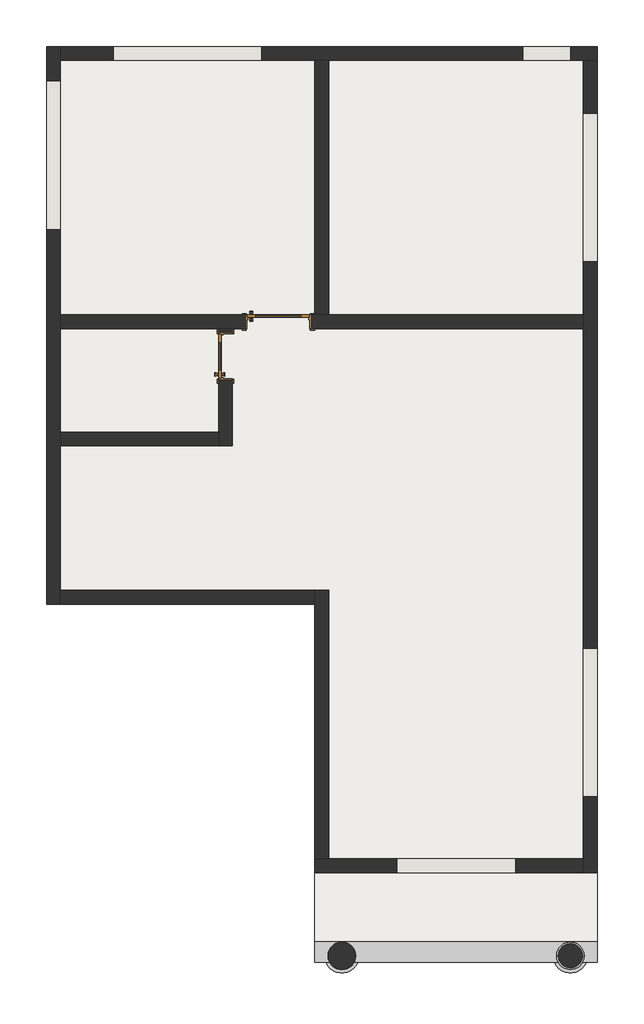
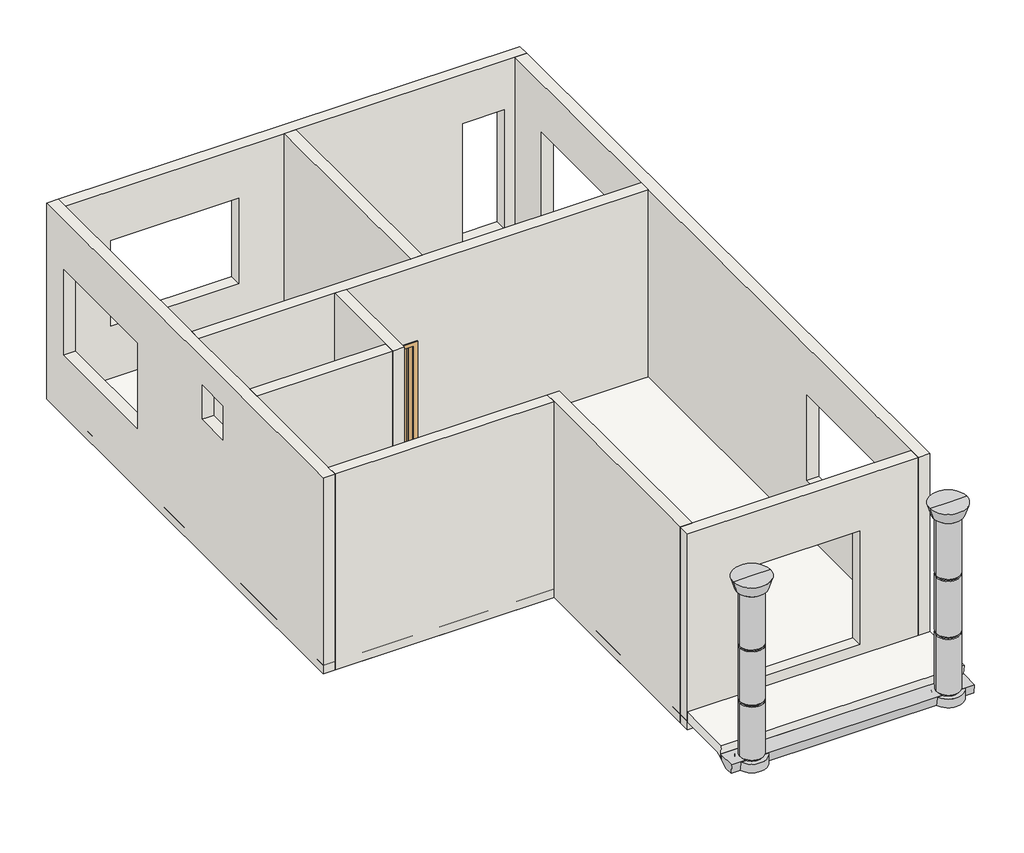
# One storey: 10 walls, 2 columns, 2 doors, 2 slabs, 1 stair flight.
"""IFC4 building model written with IfcOpenShell, lengths in millimetres."""

from ifc_helpers import new_model, si_unit, frame, origin, place, context, project, spatial, polyline, outline, extrude, faceted_brep, transform, mapped, element, save
from components import metal_clad_column_400mm_column_f648cdbd, metal_clad_column_400mm_column_d615f8bc, door_3f7a11fd, door_interior_single_5_panel_vert_wood_650_x_2100_a7f2c8da

model = new_model("IFC4")

# Units and contexts
model_context = context("Model", 3, world=origin())
ifc_project = project(units=[si_unit("LENGTHUNIT", "METRE", prefix="MILLI")], contexts=[model_context])

# Site, building, storey
site = spatial("IfcSite", under=ifc_project)
building = spatial("IfcBuilding", under=site)
storey = spatial("IfcBuildingStorey", under=building, Elevation=-100.0)

# Columns
placement = place(None, origin())
metal_clad_column_400mm_column_shape = metal_clad_column_400mm_column_f648cdbd(model_context)
element("IfcColumn", 1, ObjectType="Metal Clad Column : 400MM COLUMN", at=placement, inside=storey, context=model_context, shape_type="MappedRepresentation", body=[
    mapped(metal_clad_column_400mm_column_shape, transform((-1050.7658003, -5475.1432863, 0.0), x_axis=(1.0, 0.0, 0.0), y_axis=(0.0, 1.0, 0.0), z_axis=(0.0, 0.0, 1.0))),
])
metal_clad_column_400mm_column_2_shape = metal_clad_column_400mm_column_d615f8bc(model_context)
element("IfcColumn", 2, ObjectType="Metal Clad Column : 400MM COLUMN", at=placement, inside=storey, context=model_context, shape_type="MappedRepresentation", body=[
    mapped(metal_clad_column_400mm_column_2_shape, transform((2269.2341997, -5475.1432863, 0.0), x_axis=(-1.0, 0.0, 0.0), y_axis=(0.0, -1.0, 0.0), z_axis=(0.0, 0.0, 1.0))),
])

# Doors
door_shape = door_3f7a11fd(model_context)
element("IfcDoor", 3, ObjectType="Door-Interior-Single-5_Panel_Vert-Wood : 36\" x 82.5\"", at=placement, inside=storey, context=model_context, shape_type="MappedRepresentation", body=[
    mapped(door_shape, transform((-1973.3658003, 3738.0317137, -100.0), x_axis=(1.0, 0.0, 0.0), y_axis=(0.0, 1.0, 0.0), z_axis=(0.0, 0.0, 1.0))),
])
door_interior_single_5_panel_vert_wood_650_x_2100_shape = door_interior_single_5_panel_vert_wood_650_x_2100_a7f2c8da(model_context)
element("IfcDoor", 4, ObjectType="Door-Interior-Single-5_Panel_Vert-Wood : 650 x 2100", at=placement, inside=storey, context=model_context, shape_type="MappedRepresentation", body=[
    mapped(door_interior_single_5_panel_vert_wood_650_x_2100_shape, transform((-2743.9408003, 3234.4567137, -100.0), x_axis=(0.0, 1.0, 0.0), y_axis=(-1.0, 0.0, 0.0), z_axis=(0.0, 0.0, 1.0))),
])

# Slabs
element("IfcSlab", 5, ObjectType="6\" floor", at=placement, inside=storey, context=model_context, shape_type="SweptSolid", body=[
    extrude(outline(polyline([(-5340.7658003, 7734.8567137), (2659.2341997, 7734.8567137), (2659.2341997, -4265.1432863), (-1440.7658003, -4265.1432863), (-1440.7658003, -365.1432863), (-5340.7658003, -365.1432863), (-5340.7658003, 7734.8567137)])), frame((0.0, 0.0, -100.0), z_axis=(0.0, 0.0, 1.0), x_axis=(1.0, 0.0, 0.0)), (0.0, 0.0, 1.0), 150.0),
])
element("IfcSlab", 6, ObjectType="7\" Thickness", at=placement, inside=storey, context=model_context, shape_type="Brep", body=[
    faceted_brep([(2659.2341997, -4265.1432863, 216.6666667), (-1440.7658003, -4265.1432863, 216.6666667), (-1440.7658003, -5145.8176043, 216.6666667), (-1440.7658003, -5265.1432863, 216.6666667), (2659.2341997, -5265.1432863, 216.6666667), (2659.2341997, -5145.8176043, 216.6666667), (2659.2341997, -5246.0932863, 58.3333333), (2659.2341997, -5246.0932863, -13.2231725), (2659.2341997, -5145.8176043, 38.8666667), (2659.2341997, -4265.1432863, 38.8666667), (-1440.7658003, -4265.1432863, 38.8666667), (-1440.7658003, -5246.0932863, 58.3333333), (-1440.7658003, -5145.8176043, 38.8666667), (-1440.7658003, -5246.0932863, -13.2231725)], [[[0, 1, 2, 3, 4, 5]], [[4, 6, 7, 8, 9, 0, 5]], [[1, 0, 9, 10]], [[11, 3, 2, 1, 10, 12, 13]], [[8, 12, 10, 9]], [[4, 3, 11, 6]], [[6, 11, 13, 7]], [[12, 8, 7, 13]]]),
])

# Stair flight
element("IfcStairFlight", 7, ObjectType="3/4\" Nosing", at=placement, inside=storey, context=model_context, shape_type="Brep", body=[
    faceted_brep([(2659.2341997, -5569.9432863, 58.3333333), (-1440.7658003, -5569.9432863, 58.3333333), (-1440.7658003, -5550.8932863, -100.0), (2659.2341997, -5550.8932863, -100.0), (-1440.7658003, -5246.0932863, 58.3333333), (-1440.7658003, -5265.1432863, 58.3333333), (2659.2341997, -5265.1432863, 58.3333333), (2659.2341997, -5246.0932863, 58.3333333), (-1440.7658003, -5246.0932863, -13.2231725), (-1440.7658003, -5265.1432863, -23.1190058), (2659.2341997, -5413.1432464, -100.0), (2659.2341997, -5265.1432863, -23.1190058), (2659.2341997, -5246.0932863, -13.2231725), (-1440.7658003, -5413.1432464, -100.0)], [[[0, 1, 2, 3]], [[4, 5, 1, 0, 6, 7]], [[5, 4, 8, 9]], [[6, 0, 3, 10, 11]], [[4, 7, 12, 8]], [[3, 2, 13, 10]], [[10, 13, 9, 8, 12, 11]], [[1, 5, 9, 13, 2]], [[7, 6, 11, 12]]]),
])

# Walls
element("IfcWall", 8, ObjectType="9\" wall", at=placement, inside=storey, context=model_context, shape_type="Brep", body=[
    faceted_brep([(-5140.7658003, -365.1432863, -100.0), (-5140.7658003, -165.1432863, -100.0), (-5140.7658003, 1934.8567137, -100.0), (-5140.7658003, 2134.8567137, -100.0), (-5140.7658003, 3634.8567137, -100.0), (-5140.7658003, 3834.8567137, -100.0), (-5140.7658003, 7534.8567137, -100.0), (-5140.7658003, 7734.8567137, -100.0), (-5140.7658003, 7734.8567137, 3400.0), (-5140.7658003, 7534.8567137, 3400.0), (-5140.7658003, 3834.8567137, 3400.0), (-5140.7658003, 3634.8567137, 3400.0), (-5140.7658003, 2134.8567137, 3400.0), (-5140.7658003, 1934.8567137, 3400.0), (-5140.7658003, -165.1432863, 3400.0), (-5140.7658003, -365.1432863, 3400.0), (-5140.7658003, 7234.8567137, 2512.7), (-5140.7658003, 7234.8567137, 988.7), (-5140.7658003, 5075.8567137, 988.7), (-5140.7658003, 5075.8567137, 2512.7), (-5140.7658003, 3180.1317137, 2909.6), (-5140.7658003, 3180.1317137, 2300.0), (-5140.7658003, 2570.5317137, 2300.0), (-5140.7658003, 2570.5317137, 2909.6), (-5340.7658003, -365.1432863, -100.0), (-5340.7658003, -365.1432863, 3400.0), (-5340.7658003, 7734.8567137, 3400.0), (-5340.7658003, 7734.8567137, -100.0), (-5340.7658003, 7234.8567137, 2512.7), (-5340.7658003, 5075.8567137, 2512.7), (-5340.7658003, 5075.8567137, 988.7), (-5340.7658003, 7234.8567137, 988.7), (-5340.7658003, 3180.1317137, 2909.6), (-5340.7658003, 2570.5317137, 2909.6), (-5340.7658003, 2570.5317137, 2300.0), (-5340.7658003, 3180.1317137, 2300.0)], [[[0, 1, 2, 3, 4, 5, 6, 7, 8, 9, 10, 11, 12, 13, 14, 15], [16, 17, 18, 19], [20, 21, 22, 23]], [[24, 25, 26, 27], [28, 29, 30, 31], [32, 33, 34, 35]], [[7, 6, 5, 4, 3, 2, 1, 0, 24, 27]], [[15, 14, 13, 12, 11, 10, 9, 8, 26, 25]], [[8, 7, 27, 26]], [[0, 15, 25, 24]], [[17, 16, 28, 31]], [[18, 17, 31, 30]], [[19, 18, 30, 29]], [[16, 19, 29, 28]], [[21, 20, 32, 35]], [[22, 21, 35, 34]], [[23, 22, 34, 33]], [[20, 23, 33, 32]]]),
])
element("IfcWall", 9, ObjectType="9\" wall", at=placement, inside=storey, context=model_context, shape_type="Brep", body=[
    faceted_brep([(-5140.7658003, 7534.8567137, -100.0), (-1440.7658003, 7534.8567137, -100.0), (-1240.7658003, 7534.8567137, -100.0), (2459.2341997, 7534.8567137, -100.0), (2659.2341997, 7534.8567137, -100.0), (2659.2341997, 7534.8567137, 3400.0), (2459.2341997, 7534.8567137, 3400.0), (-1240.7658003, 7534.8567137, 3400.0), (-1440.7658003, 7534.8567137, 3400.0), (-5140.7658003, 7534.8567137, 3400.0), (2277.0341997, 7534.8567137, 2525.4), (2277.0341997, 7534.8567137, 400.0), (1576.2341997, 7534.8567137, 400.0), (1576.2341997, 7534.8567137, 2525.4), (-2211.2658003, 7534.8567137, 2512.7), (-2211.2658003, 7534.8567137, 988.7), (-4370.2658003, 7534.8567137, 988.7), (-4370.2658003, 7534.8567137, 2512.7), (2659.2341997, 7734.8567137, -100.0), (-5140.7658003, 7734.8567137, -100.0), (-5140.7658003, 7734.8567137, 3400.0), (2659.2341997, 7734.8567137, 3400.0), (2277.0341997, 7734.8567137, 400.0), (2277.0341997, 7734.8567137, 2525.4), (1576.2341997, 7734.8567137, 2525.4), (1576.2341997, 7734.8567137, 400.0), (-2211.2658003, 7734.8567137, 2512.7), (-4370.2658003, 7734.8567137, 2512.7), (-4370.2658003, 7734.8567137, 988.7), (-2211.2658003, 7734.8567137, 988.7)], [[[0, 1, 2, 3, 4, 5, 6, 7, 8, 9], [10, 11, 12, 13], [14, 15, 16, 17]], [[18, 19, 20, 21], [22, 23, 24, 25], [26, 27, 28, 29]], [[4, 3, 2, 1, 0, 19, 18]], [[9, 8, 7, 6, 5, 21, 20]], [[0, 9, 20, 19]], [[5, 4, 18, 21]], [[22, 11, 10, 23]], [[23, 10, 13, 24]], [[24, 13, 12, 25]], [[11, 22, 25, 12]], [[15, 14, 26, 29]], [[16, 15, 29, 28]], [[17, 16, 28, 27]], [[14, 17, 27, 26]]]),
])
element("IfcWall", 10, ObjectType="9\" wall", at=placement, inside=storey, context=model_context, shape_type="Brep", body=[
    faceted_brep([(2459.2341997, 7534.8567137, -100.0), (2459.2341997, 3834.8567137, -100.0), (2459.2341997, 3634.8567137, -100.0), (2459.2341997, -4065.1432863, -100.0), (2459.2341997, -4265.1432863, -100.0), (2459.2341997, -4265.1432863, 3400.0), (2459.2341997, -4065.1432863, 3400.0), (2459.2341997, 3634.8567137, 3400.0), (2459.2341997, 3834.8567137, 3400.0), (2459.2341997, 7534.8567137, 3400.0), (2459.2341997, -3165.1432863, 2538.1), (2459.2341997, -3165.1432863, 1014.1), (2459.2341997, -1006.1432863, 1014.1), (2459.2341997, -1006.1432863, 2538.1), (2459.2341997, 4605.3567137, 2525.4), (2459.2341997, 4605.3567137, 1001.4), (2459.2341997, 6764.3567137, 1001.4), (2459.2341997, 6764.3567137, 2525.4), (2659.2341997, 7534.8567137, -100.0), (2659.2341997, 7534.8567137, 3400.0), (2659.2341997, -4265.1432863, 3400.0), (2659.2341997, -4265.1432863, -100.0), (2659.2341997, -3165.1432863, 2538.1), (2659.2341997, -1006.1432863, 2538.1), (2659.2341997, -1006.1432863, 1014.1), (2659.2341997, -3165.1432863, 1014.1), (2659.2341997, 4605.3567137, 2525.4), (2659.2341997, 6764.3567137, 2525.4), (2659.2341997, 6764.3567137, 1001.4), (2659.2341997, 4605.3567137, 1001.4)], [[[0, 1, 2, 3, 4, 5, 6, 7, 8, 9], [10, 11, 12, 13], [14, 15, 16, 17]], [[18, 19, 20, 21], [22, 23, 24, 25], [26, 27, 28, 29]], [[4, 3, 2, 1, 0, 18, 21]], [[9, 8, 7, 6, 5, 20, 19]], [[0, 9, 19, 18]], [[5, 4, 21, 20]], [[11, 10, 22, 25]], [[12, 11, 25, 24]], [[13, 12, 24, 23]], [[10, 13, 23, 22]], [[15, 14, 26, 29]], [[16, 15, 29, 28]], [[17, 16, 28, 27]], [[14, 17, 27, 26]]]),
])
element("IfcWall", 11, ObjectType="9\" wall", at=placement, inside=storey, context=model_context, shape_type="Brep", body=[
    faceted_brep([(2459.2341997, -4065.1432863, -100.0), (-1240.7658003, -4065.1432863, -100.0), (-1440.7658003, -4065.1432863, -100.0), (-1440.7658003, -4065.1432863, 3400.0), (-1240.7658003, -4065.1432863, 3400.0), (2459.2341997, -4065.1432863, 3400.0), (1472.8341997, -4065.1432863, 2432.0), (-254.3658003, -4065.1432863, 2432.0), (-254.3658003, -4065.1432863, 400.0), (1472.8341997, -4065.1432863, 400.0), (2459.2341997, -4265.1432863, -100.0), (2459.2341997, -4265.1432863, 3400.0), (-1440.7658003, -4265.1432863, 3400.0), (-1440.7658003, -4265.1432863, -100.0), (1472.8341997, -4265.1432863, 2432.0), (1472.8341997, -4265.1432863, 400.0), (-254.3658003, -4265.1432863, 400.0), (-254.3658003, -4265.1432863, 2432.0)], [[[0, 1, 2, 3, 4, 5], [6, 7, 8, 9]], [[10, 11, 12, 13], [14, 15, 16, 17]], [[2, 1, 0, 10, 13]], [[5, 4, 3, 12, 11]], [[0, 5, 11, 10]], [[3, 2, 13, 12]], [[15, 14, 6, 9]], [[16, 15, 9, 8]], [[17, 16, 8, 7]], [[14, 17, 7, 6]]]),
])
element("IfcWall", 12, ObjectType="9\" wall", at=placement, inside=storey, context=model_context, shape_type="Brep", body=[
    faceted_brep([(-1440.7658003, -165.1432863, -100.0), (-1440.7658003, -365.1432863, -100.0), (-1440.7658003, -4065.1432863, -100.0), (-1440.7658003, -4065.1432863, 3400.0), (-1440.7658003, -365.1432863, 3400.0), (-1440.7658003, -165.1432863, 3400.0), (-1240.7658003, -165.1432863, -100.0), (-1240.7658003, -165.1432863, 3400.0), (-1240.7658003, -4065.1432863, 3400.0), (-1240.7658003, -4065.1432863, -100.0)], [[[0, 1, 2, 3, 4, 5]], [[6, 7, 8, 9]], [[2, 1, 0, 6, 9]], [[5, 4, 3, 8, 7]], [[0, 5, 7, 6]], [[3, 2, 9, 8]]]),
])
element("IfcWall", 13, ObjectType="9\" wall", at=placement, inside=storey, context=model_context, shape_type="Brep", body=[
    faceted_brep([(2459.2341997, 3634.8567137, 3400.0), (-2640.7658003, 3634.8567137, 3400.0), (-2840.7658003, 3634.8567137, 3400.0), (-5140.7658003, 3634.8567137, 3400.0), (-5140.7658003, 3634.8567137, -100.0), (-2840.7658003, 3634.8567137, -100.0), (-2640.7658003, 3634.8567137, -100.0), (-2455.9658003, 3634.8567137, -100.0), (-2455.9658003, 3634.8567137, 2025.4), (-1490.7658003, 3634.8567137, 2025.4), (-1490.7658003, 3634.8567137, -100.0), (2459.2341997, 3634.8567137, -100.0), (-5140.7658003, 3834.8567137, 3400.0), (-1440.7658003, 3834.8567137, 3400.0), (-1240.7658003, 3834.8567137, 3400.0), (2459.2341997, 3834.8567137, 3400.0), (2459.2341997, 3834.8567137, -100.0), (-1240.7658003, 3834.8567137, -100.0), (-1440.7658003, 3834.8567137, -100.0), (-1490.7658003, 3834.8567137, -100.0), (-1490.7658003, 3834.8567137, 2025.4), (-2455.9658003, 3834.8567137, 2025.4), (-2455.9658003, 3834.8567137, -100.0), (-5140.7658003, 3834.8567137, -100.0)], [[[0, 1, 2, 3, 4, 5, 6, 7, 8, 9, 10, 11]], [[12, 13, 14, 15, 16, 17, 18, 19, 20, 21, 22, 23]], [[4, 23, 22, 7, 6, 5]], [[16, 11, 10, 19, 18, 17]], [[3, 2, 1, 0, 15, 14, 13, 12]], [[4, 3, 12, 23]], [[0, 11, 16, 15]], [[9, 20, 19, 10]], [[20, 9, 8, 21]], [[21, 8, 7, 22]]]),
])
element("IfcWall", 14, ObjectType="9\" wall", at=placement, inside=storey, context=model_context, shape_type="SweptSolid", body=[
    extrude(outline(polyline([(-1440.7658003, -365.1432863), (-5140.7658003, -365.1432863), (-5140.7658003, -165.1432863), (-1440.7658003, -165.1432863), (-1440.7658003, -365.1432863)])), frame((0.0, 0.0, -100.0), z_axis=(0.0, 0.0, 1.0), x_axis=(1.0, 0.0, 0.0)), (0.0, 0.0, 1.0), 3500.0),
])
element("IfcWall", 15, ObjectType="9\" wall", at=placement, inside=storey, context=model_context, shape_type="SweptSolid", body=[
    extrude(outline(polyline([(-1440.7658003, 3834.8567137), (-1440.7658003, 7534.8567137), (-1240.7658003, 7534.8567137), (-1240.7658003, 3834.8567137), (-1440.7658003, 3834.8567137)])), frame((0.0, 0.0, -100.0), z_axis=(0.0, 0.0, 1.0), x_axis=(1.0, 0.0, 0.0)), (0.0, 0.0, 1.0), 3500.0),
])
element("IfcWall", 16, ObjectType="9\" wall", at=placement, inside=storey, context=model_context, shape_type="Brep", body=[
    faceted_brep([(-2840.7658003, 1934.8567137, 3400.0), (-2840.7658003, 2134.8567137, 3400.0), (-2840.7658003, 3634.8567137, 3400.0), (-2840.7658003, 3634.8567137, -100.0), (-2840.7658003, 3584.8567137, -100.0), (-2840.7658003, 3584.8567137, 2025.4), (-2840.7658003, 2884.0567137, 2025.4), (-2840.7658003, 2884.0567137, -100.0), (-2840.7658003, 2134.8567137, -100.0), (-2840.7658003, 1934.8567137, -100.0), (-2640.7658003, 3634.8567137, 3400.0), (-2640.7658003, 1934.8567137, 3400.0), (-2640.7658003, 1934.8567137, -100.0), (-2640.7658003, 2884.0567137, -100.0), (-2640.7658003, 2884.0567137, 2025.4), (-2640.7658003, 3584.8567137, 2025.4), (-2640.7658003, 3584.8567137, -100.0), (-2640.7658003, 3634.8567137, -100.0)], [[[0, 1, 2, 3, 4, 5, 6, 7, 8, 9]], [[10, 11, 12, 13, 14, 15, 16, 17]], [[3, 17, 16, 4]], [[12, 9, 8, 7, 13]], [[2, 1, 0, 11, 10]], [[3, 2, 10, 17]], [[0, 9, 12, 11]], [[15, 5, 4, 16]], [[5, 15, 14, 6]], [[6, 14, 13, 7]]]),
])
element("IfcWall", 17, ObjectType="9\" wall", at=placement, inside=storey, context=model_context, shape_type="SweptSolid", body=[
    extrude(outline(polyline([(-5140.7658003, 2134.8567137), (-2840.7658003, 2134.8567137), (-2840.7658003, 1934.8567137), (-5140.7658003, 1934.8567137), (-5140.7658003, 2134.8567137)])), frame((0.0, 0.0, -100.0), z_axis=(0.0, 0.0, 1.0), x_axis=(1.0, 0.0, 0.0)), (0.0, 0.0, 1.0), 3500.0),
])

save(model, "model.ifc")

# Revit data of these elements
# Grids (mm)
#   "1": line (5455.554, 7734.857) -> (-7758.78, 7734.857)
#   "A": line (-5340.766, 9128.599) -> (-5340.766, -7602.671)
#   "B": line (-1340.766, 9128.599) -> (-1340.766, -7602.671)
#   "2": line (5455.554, 3734.857) -> (-7758.78, 3734.857)
#   "3": line (5455.554, -265.143) -> (-7758.78, -265.143)
#   "4": line (5455.554, -4165.143) -> (-7758.78, -4165.143)
#   "C": line (2659.234, 9128.599) -> (2659.234, -7602.671)
# Type "Metal Clad Column : 400MM COLUMN"
#   Assembly Code = "B1010200"
#   Base = 0' - 6"
#   Capital = 0' - 8"
#   Diameter = 1' - 3.74803"
#   Joint Depth = 0' - 1"
#   Joint Width = 0' - 1 1/2"
#   Offset base level = 0' - 0"
#   Offset top level = 0' - 0"
#   Material = Aluminum
# Type "Door-Interior-Single-5_Panel_Vert-Wood : 36\" x 82.5\""
#   Type Mark = "20"
#   Assembly Code = "C1020300"
#   Analytic Construction = "Wooden"
#   Top Rail = 0' - 4 11/16"
#   Thickness = 0' - 1 3/8"
#   Thermal Resistance (R) = 2.5876 (h·ft²·°F)/BTU
#   Swing Angle [instance default] = 90.00°
#   Stiles = 0' - 4 3/4"
#   Rough Width = 3' - 2"
#   Rough Height = 6' - 11.67717"
#   Intermediate Rail = 0' - 4 1/2"
#   Height = 6' - 10.67717"
#   Width = 3' - 0"
#   Heat Transfer Coefficient (U) = 0.3865 BTU/(h·ft²·°F)
#   Bottom Rail = 0' - 9 1/8"
#   Trim Material = Cherry
#   Panel Material = Cherry
#   Frame Material = Cherry
#   Door Handle Material = Aluminum
#   Visual Light Transmittance = 0
#   Solar Heat Gain Coefficient = 0
#   Wall Closure = (empty or 0)
#   Function = (empty or 0)
# Type "Door-Interior-Single-5_Panel_Vert-Wood : 650 x 2100"
#   Type Mark = "22"
#   Assembly Code = "C1020300"
#   Analytic Construction = "Wooden"
#   Top Rail = 0' - 4 11/16"
#   Thickness = 0' - 1 3/8"
#   Thermal Resistance (R) = 2.5876 (h·ft²·°F)/BTU
#   Swing Angle [instance default] = 90.00°
#   Stiles = 0' - 4 3/4"
#   Rough Width = 2' - 3.59055"
#   Rough Height = 6' - 11.67717"
#   Intermediate Rail = 0' - 4 1/2"
#   Height = 6' - 10.67717"
#   Width = 2' - 1.59055"
#   Heat Transfer Coefficient (U) = 0.3865 BTU/(h·ft²·°F)
#   Bottom Rail = 0' - 9 1/8"
#   Trim Material = Cherry
#   Panel Material = Cherry
#   Frame Material = Cherry
#   Door Handle Material = Aluminum
#   Visual Light Transmittance = 0
#   Solar Heat Gain Coefficient = 0
#   Wall Closure = (empty or 0)
#   Function = (empty or 0)
# Type "6\" floor"
#   Assembly Code = "B1010"
#   Function = 0
#   Layers, outside or top first: 0' - 5.90551" "MATERIAL -WHITE" (function 1)
# Type "9\" wall"
#   Assembly Code = "B2010"
#   Layers, outside or top first: 0' - 7.87402" "MATERIAL -WHITE" (function 1)
# Elements 1, 2 (IfcColumn, "Metal Clad Column : 400MM COLUMN")
#   Phase Created = New Construction
#   Materials on its faces: "Aluminum"
# Element 3 (IfcDoor, "Door-Interior-Single-5_Panel_Vert-Wood : 36\" x 82.5\"")
#   Phase Created = New Construction
#   Materials on its faces: "Cherry", "Aluminum"
# Element 4 (IfcDoor, "Door-Interior-Single-5_Panel_Vert-Wood : 650 x 2100")
#   Swing Angle = 90.00°
#   Phase Created = New Construction
#   Materials on its faces: "Cherry", "Aluminum"
# Element 5 (IfcSlab, "6\" floor")
#   built-in parameter 1001955 = 3.14159 (stored number, unit not read)
#   Height Offset From Level = 0' - 5.90551"
#   Phase Created = New Construction
#   Materials on its faces: "MATERIAL -WHITE"
# Element 6 (IfcSlab, "7\" Thickness")
#   Phase Created = New Construction
#   Materials on its faces: "Concrete, Cast-in-Place gray"
# Element 7 (IfcStairFlight, "3/4\" Nosing")
#   Phase Created = New Construction
#   Materials on its faces: "Concrete, Cast-in-Place gray"
# Elements 8, 9, 10, 11, 12, 13, 14, 15, 16, 17 (IfcWall, "9\" wall")
#   Top Offset = 0' - 0"
#   Base Offset = 0' - 0"
#   wall height = 11' - 5.79528"
#   Phase Created = New Construction
#   Materials on its faces: "MATERIAL -WHITE"
# Materials
#   "Aluminum": class "Metal", colour RGB 247 247 247, transparency 0, Description = "Aluminum 6061", Cost = 0
#   "Cherry": class "Wood", colour RGB 226 177 128, transparency 0, Description = "Prunus Serotina", Cost = 0
#   "MATERIAL -WHITE": class "Generic", colour RGB 255 255 255, transparency 0, Cost = 0
#   "Concrete, Cast-in-Place gray": class "Concrete", colour RGB 192 192 192, transparency 0, Description = "Cast-in-place concrete", Cost = 0
